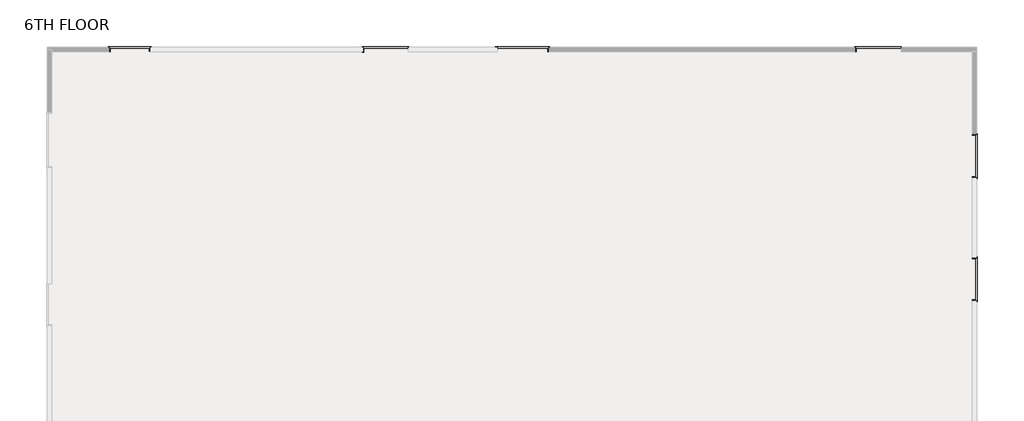
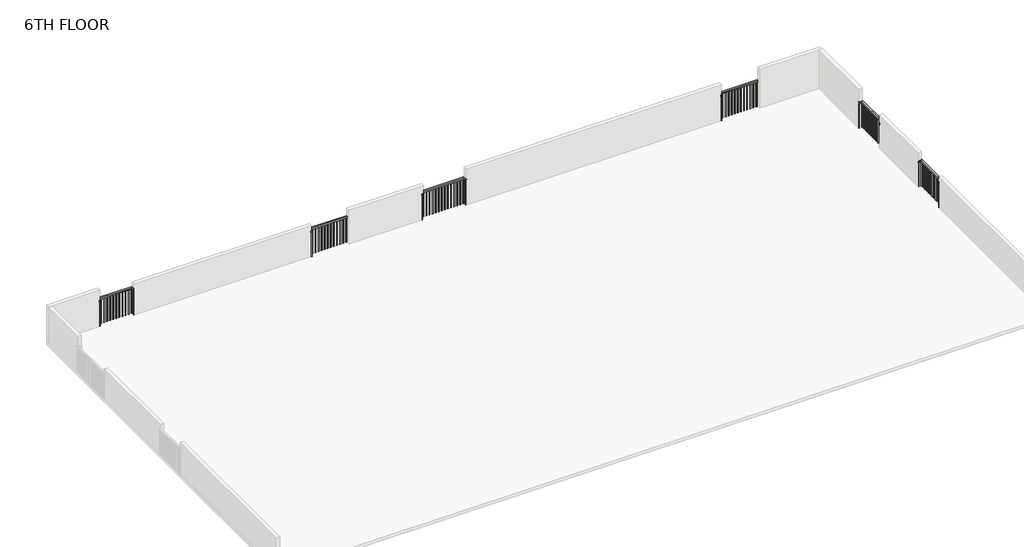
# One storey, part 3 of 3: 6 railings.
"""IFC4 building model written with IfcOpenShell, lengths in millimetres."""

from ifc_helpers import new_model, si_unit, frame, origin, place, context, project, spatial, polyline, outline, extrude, faceted_brep, element, save

model = new_model("IFC4")

# Units and contexts
model_context = context("Model", 3, world=origin())
ifc_project = project(units=[si_unit("LENGTHUNIT", "METRE", prefix="MILLI")], contexts=[model_context])

# Site, building, storey
site = spatial("IfcSite", under=ifc_project)
building = spatial("IfcBuilding", under=site)
storey = spatial("IfcBuildingStorey", under=building, Name="6TH FLOOR", Elevation=19202.4)

# Railings
placement = place(None, origin())
element("IfcRailing", 1, ObjectType="Handrail - Rectangular", at=placement, inside=storey, context=model_context, shape_type="SolidModel", body=[
    faceted_brep([(-11412.4067989, 8355.7067329, 20116.8), (-11412.4067989, 8355.7067329, 20066.0), (-11361.6067989, 8355.7067329, 20066.0), (-11361.6067989, 8355.7067329, 20116.8), (-11412.4067989, 8495.4067329, 20116.8), (-11412.4067989, 8495.4067329, 20066.0), (-11361.6067989, 8444.6067329, 20066.0), (-11361.6067989, 8444.6067329, 20116.8), (-10231.3067989, 8495.4067329, 20116.8), (-10231.3067989, 8495.4067329, 20066.0), (-10282.1067989, 8444.6067329, 20066.0), (-10282.1067989, 8444.6067329, 20116.8), (-10231.3067989, 8368.4067329, 20116.8), (-10282.1067989, 8368.4067329, 20116.8), (-10282.1067989, 8368.4067329, 20066.0), (-10231.3067989, 8368.4067329, 20066.0)], [[[0, 1, 2, 3]], [[1, 0, 4, 5]], [[2, 1, 5, 6]], [[3, 2, 6, 7]], [[0, 3, 7, 4]], [[5, 4, 8, 9]], [[6, 5, 9, 10]], [[7, 6, 10, 11]], [[4, 7, 11, 8]], [[12, 13, 14, 15]], [[9, 8, 12, 15]], [[10, 9, 15, 14]], [[11, 10, 14, 13]], [[8, 11, 13, 12]]]),
    extrude(outline(polyline([(-10278.9317989, 8460.4817329), (-10278.9317989, 8479.5317329), (-10259.8817989, 8479.5317329), (-10259.8817989, 8460.4817329), (-10278.9317989, 8460.4817329)])), frame((0.0, 0.0, 19202.4), z_axis=(0.0, 0.0, 1.0), x_axis=(1.0, 0.0, 0.0)), (0.0, 0.0, 1.0), 863.6),
    extrude(outline(polyline([(-10380.5317989, 8460.4817329), (-10380.5317989, 8479.5317329), (-10361.4817989, 8479.5317329), (-10361.4817989, 8460.4817329), (-10380.5317989, 8460.4817329)])), frame((0.0, 0.0, 19202.4), z_axis=(0.0, 0.0, 1.0), x_axis=(1.0, 0.0, 0.0)), (0.0, 0.0, 1.0), 863.6),
    extrude(outline(polyline([(-10482.1317989, 8460.4817329), (-10482.1317989, 8479.5317329), (-10463.0817989, 8479.5317329), (-10463.0817989, 8460.4817329), (-10482.1317989, 8460.4817329)])), frame((0.0, 0.0, 19202.4), z_axis=(0.0, 0.0, 1.0), x_axis=(1.0, 0.0, 0.0)), (0.0, 0.0, 1.0), 863.6),
    extrude(outline(polyline([(-10583.7317989, 8460.4817329), (-10583.7317989, 8479.5317329), (-10564.6817989, 8479.5317329), (-10564.6817989, 8460.4817329), (-10583.7317989, 8460.4817329)])), frame((0.0, 0.0, 19202.4), z_axis=(0.0, 0.0, 1.0), x_axis=(1.0, 0.0, 0.0)), (0.0, 0.0, 1.0), 863.6),
    extrude(outline(polyline([(-10685.3317989, 8460.4817329), (-10685.3317989, 8479.5317329), (-10666.2817989, 8479.5317329), (-10666.2817989, 8460.4817329), (-10685.3317989, 8460.4817329)])), frame((0.0, 0.0, 19202.4), z_axis=(0.0, 0.0, 1.0), x_axis=(1.0, 0.0, 0.0)), (0.0, 0.0, 1.0), 863.6),
    extrude(outline(polyline([(-10786.9317989, 8460.4817329), (-10786.9317989, 8479.5317329), (-10767.8817989, 8479.5317329), (-10767.8817989, 8460.4817329), (-10786.9317989, 8460.4817329)])), frame((0.0, 0.0, 19202.4), z_axis=(0.0, 0.0, 1.0), x_axis=(1.0, 0.0, 0.0)), (0.0, 0.0, 1.0), 863.6),
    extrude(outline(polyline([(-10888.5317989, 8460.4817329), (-10888.5317989, 8479.5317329), (-10869.4817989, 8479.5317329), (-10869.4817989, 8460.4817329), (-10888.5317989, 8460.4817329)])), frame((0.0, 0.0, 19202.4), z_axis=(0.0, 0.0, 1.0), x_axis=(1.0, 0.0, 0.0)), (0.0, 0.0, 1.0), 863.6),
    extrude(outline(polyline([(-10990.1317989, 8460.4817329), (-10990.1317989, 8479.5317329), (-10971.0817989, 8479.5317329), (-10971.0817989, 8460.4817329), (-10990.1317989, 8460.4817329)])), frame((0.0, 0.0, 19202.4), z_axis=(0.0, 0.0, 1.0), x_axis=(1.0, 0.0, 0.0)), (0.0, 0.0, 1.0), 863.6),
    extrude(outline(polyline([(-11091.7317989, 8460.4817329), (-11091.7317989, 8479.5317329), (-11072.6817989, 8479.5317329), (-11072.6817989, 8460.4817329), (-11091.7317989, 8460.4817329)])), frame((0.0, 0.0, 19202.4), z_axis=(0.0, 0.0, 1.0), x_axis=(1.0, 0.0, 0.0)), (0.0, 0.0, 1.0), 863.6),
    extrude(outline(polyline([(-11193.3317989, 8460.4817329), (-11193.3317989, 8479.5317329), (-11174.2817989, 8479.5317329), (-11174.2817989, 8460.4817329), (-11193.3317989, 8460.4817329)])), frame((0.0, 0.0, 19202.4), z_axis=(0.0, 0.0, 1.0), x_axis=(1.0, 0.0, 0.0)), (0.0, 0.0, 1.0), 863.6),
    extrude(outline(polyline([(-11294.9317989, 8460.4817329), (-11294.9317989, 8479.5317329), (-11275.8817989, 8479.5317329), (-11275.8817989, 8460.4817329), (-11294.9317989, 8460.4817329)])), frame((0.0, 0.0, 19202.4), z_axis=(0.0, 0.0, 1.0), x_axis=(1.0, 0.0, 0.0)), (0.0, 0.0, 1.0), 863.6),
    extrude(outline(polyline([(-11377.4817989, 8447.7817329), (-11396.5317989, 8447.7817329), (-11396.5317989, 8466.8317329), (-11377.4817989, 8466.8317329), (-11377.4817989, 8447.7817329)])), frame((0.0, 0.0, 19202.4), z_axis=(0.0, 0.0, 1.0), x_axis=(1.0, 0.0, 0.0)), (0.0, 0.0, 1.0), 863.6),
    extrude(outline(polyline([(-10266.2317989, 8460.4817329), (-10266.2317989, 8479.5317329), (-10247.1817989, 8479.5317329), (-10247.1817989, 8460.4817329), (-10266.2317989, 8460.4817329)])), frame((0.0, 0.0, 19202.4), z_axis=(0.0, 0.0, 1.0), x_axis=(1.0, 0.0, 0.0)), (0.0, 0.0, 1.0), 863.6),
    extrude(outline(polyline([(-11377.4817989, 8460.4817329), (-11396.5317989, 8460.4817329), (-11396.5317989, 8479.5317329), (-11377.4817989, 8479.5317329), (-11377.4817989, 8460.4817329)])), frame((0.0, 0.0, 19202.4), z_axis=(0.0, 0.0, 1.0), x_axis=(1.0, 0.0, 0.0)), (0.0, 0.0, 1.0), 863.6),
    extrude(outline(polyline([(-10266.2317989, 8387.4567329), (-10247.1817989, 8387.4567329), (-10247.1817989, 8368.4067329), (-10266.2317989, 8368.4067329), (-10266.2317989, 8387.4567329)])), frame((0.0, 0.0, 19202.4), z_axis=(0.0, 0.0, 1.0), x_axis=(1.0, 0.0, 0.0)), (0.0, 0.0, 1.0), 863.6),
    extrude(outline(polyline([(-11377.4817989, 8355.7067329), (-11396.5317989, 8355.7067329), (-11396.5317989, 8374.7567329), (-11377.4817989, 8374.7567329), (-11377.4817989, 8355.7067329)])), frame((0.0, 0.0, 19202.4), z_axis=(0.0, 0.0, 1.0), x_axis=(1.0, 0.0, 0.0)), (0.0, 0.0, 1.0), 863.6),
])
element("IfcRailing", 2, ObjectType="Handrail - Rectangular", at=placement, inside=storey, context=model_context, shape_type="SolidModel", body=[
    faceted_brep([(-4407.8487992, 8336.6567329, 20116.8), (-4407.8487992, 8336.6567329, 20066.0), (-4357.0487992, 8336.6567329, 20066.0), (-4357.0487992, 8336.6567329, 20116.8), (-4407.8487992, 8495.4067329, 20116.8), (-4407.8487992, 8495.4067329, 20066.0), (-4357.0487992, 8444.6067329, 20066.0), (-4357.0487992, 8444.6067329, 20116.8), (-3120.4490672, 8495.4067329, 20116.8), (-3120.4490672, 8444.6067329, 20116.8), (-3120.4490672, 8444.6067329, 20066.0), (-3120.4490672, 8495.4067329, 20066.0)], [[[0, 1, 2, 3]], [[1, 0, 4, 5]], [[2, 1, 5, 6]], [[3, 2, 6, 7]], [[0, 3, 7, 4]], [[8, 9, 10, 11]], [[5, 4, 8, 11]], [[6, 5, 11, 10]], [[7, 6, 10, 9]], [[4, 7, 9, 8]]]),
    extrude(outline(polyline([(-3172.7737992, 8460.4817329), (-3172.7737992, 8479.5317329), (-3153.7237992, 8479.5317329), (-3153.7237992, 8460.4817329), (-3172.7737992, 8460.4817329)])), frame((0.0, 0.0, 19202.4), z_axis=(0.0, 0.0, 1.0), x_axis=(1.0, 0.0, 0.0)), (0.0, 0.0, 1.0), 863.6),
    extrude(outline(polyline([(-3274.3737992, 8460.4817329), (-3274.3737992, 8479.5317329), (-3255.3237992, 8479.5317329), (-3255.3237992, 8460.4817329), (-3274.3737992, 8460.4817329)])), frame((0.0, 0.0, 19202.4), z_axis=(0.0, 0.0, 1.0), x_axis=(1.0, 0.0, 0.0)), (0.0, 0.0, 1.0), 863.6),
    extrude(outline(polyline([(-3375.9737992, 8460.4817329), (-3375.9737992, 8479.5317329), (-3356.9237992, 8479.5317329), (-3356.9237992, 8460.4817329), (-3375.9737992, 8460.4817329)])), frame((0.0, 0.0, 19202.4), z_axis=(0.0, 0.0, 1.0), x_axis=(1.0, 0.0, 0.0)), (0.0, 0.0, 1.0), 863.6),
    extrude(outline(polyline([(-3477.5737992, 8460.4817329), (-3477.5737992, 8479.5317329), (-3458.5237992, 8479.5317329), (-3458.5237992, 8460.4817329), (-3477.5737992, 8460.4817329)])), frame((0.0, 0.0, 19202.4), z_axis=(0.0, 0.0, 1.0), x_axis=(1.0, 0.0, 0.0)), (0.0, 0.0, 1.0), 863.6),
    extrude(outline(polyline([(-3579.1737992, 8460.4817329), (-3579.1737992, 8479.5317329), (-3560.1237992, 8479.5317329), (-3560.1237992, 8460.4817329), (-3579.1737992, 8460.4817329)])), frame((0.0, 0.0, 19202.4), z_axis=(0.0, 0.0, 1.0), x_axis=(1.0, 0.0, 0.0)), (0.0, 0.0, 1.0), 863.6),
    extrude(outline(polyline([(-3680.7737992, 8460.4817329), (-3680.7737992, 8479.5317329), (-3661.7237992, 8479.5317329), (-3661.7237992, 8460.4817329), (-3680.7737992, 8460.4817329)])), frame((0.0, 0.0, 19202.4), z_axis=(0.0, 0.0, 1.0), x_axis=(1.0, 0.0, 0.0)), (0.0, 0.0, 1.0), 863.6),
    extrude(outline(polyline([(-3782.3737992, 8460.4817329), (-3782.3737992, 8479.5317329), (-3763.3237992, 8479.5317329), (-3763.3237992, 8460.4817329), (-3782.3737992, 8460.4817329)])), frame((0.0, 0.0, 19202.4), z_axis=(0.0, 0.0, 1.0), x_axis=(1.0, 0.0, 0.0)), (0.0, 0.0, 1.0), 863.6),
    extrude(outline(polyline([(-3883.9737992, 8460.4817329), (-3883.9737992, 8479.5317329), (-3864.9237992, 8479.5317329), (-3864.9237992, 8460.4817329), (-3883.9737992, 8460.4817329)])), frame((0.0, 0.0, 19202.4), z_axis=(0.0, 0.0, 1.0), x_axis=(1.0, 0.0, 0.0)), (0.0, 0.0, 1.0), 863.6),
    extrude(outline(polyline([(-3985.5737992, 8460.4817329), (-3985.5737992, 8479.5317329), (-3966.5237992, 8479.5317329), (-3966.5237992, 8460.4817329), (-3985.5737992, 8460.4817329)])), frame((0.0, 0.0, 19202.4), z_axis=(0.0, 0.0, 1.0), x_axis=(1.0, 0.0, 0.0)), (0.0, 0.0, 1.0), 863.6),
    extrude(outline(polyline([(-4087.1737992, 8460.4817329), (-4087.1737992, 8479.5317329), (-4068.1237992, 8479.5317329), (-4068.1237992, 8460.4817329), (-4087.1737992, 8460.4817329)])), frame((0.0, 0.0, 19202.4), z_axis=(0.0, 0.0, 1.0), x_axis=(1.0, 0.0, 0.0)), (0.0, 0.0, 1.0), 863.6),
    extrude(outline(polyline([(-4188.7737992, 8460.4817329), (-4188.7737992, 8479.5317329), (-4169.7237992, 8479.5317329), (-4169.7237992, 8460.4817329), (-4188.7737992, 8460.4817329)])), frame((0.0, 0.0, 19202.4), z_axis=(0.0, 0.0, 1.0), x_axis=(1.0, 0.0, 0.0)), (0.0, 0.0, 1.0), 863.6),
    extrude(outline(polyline([(-4290.3737992, 8460.4817329), (-4290.3737992, 8479.5317329), (-4271.3237992, 8479.5317329), (-4271.3237992, 8460.4817329), (-4290.3737992, 8460.4817329)])), frame((0.0, 0.0, 19202.4), z_axis=(0.0, 0.0, 1.0), x_axis=(1.0, 0.0, 0.0)), (0.0, 0.0, 1.0), 863.6),
    extrude(outline(polyline([(-4372.9237992, 8428.7317329), (-4391.9737992, 8428.7317329), (-4391.9737992, 8447.7817329), (-4372.9237992, 8447.7817329), (-4372.9237992, 8428.7317329)])), frame((0.0, 0.0, 19202.4), z_axis=(0.0, 0.0, 1.0), x_axis=(1.0, 0.0, 0.0)), (0.0, 0.0, 1.0), 863.6),
    extrude(outline(polyline([(-4372.9237992, 8460.4817329), (-4391.9737992, 8460.4817329), (-4391.9737992, 8479.5317329), (-4372.9237992, 8479.5317329), (-4372.9237992, 8460.4817329)])), frame((0.0, 0.0, 19202.4), z_axis=(0.0, 0.0, 1.0), x_axis=(1.0, 0.0, 0.0)), (0.0, 0.0, 1.0), 863.6),
    extrude(outline(polyline([(-3139.4990672, 8460.4817329), (-3139.4990672, 8479.5317329), (-3120.4490672, 8479.5317329), (-3120.4490672, 8460.4817329), (-3139.4990672, 8460.4817329)])), frame((0.0, 0.0, 19202.4), z_axis=(0.0, 0.0, 1.0), x_axis=(1.0, 0.0, 0.0)), (0.0, 0.0, 1.0), 863.6),
    extrude(outline(polyline([(-4372.9237992, 8336.6567329), (-4391.9737992, 8336.6567329), (-4391.9737992, 8355.7067329), (-4372.9237992, 8355.7067329), (-4372.9237992, 8336.6567329)])), frame((0.0, 0.0, 19202.4), z_axis=(0.0, 0.0, 1.0), x_axis=(1.0, 0.0, 0.0)), (0.0, 0.0, 1.0), 863.6),
])
element("IfcRailing", 3, ObjectType="Handrail - Rectangular", at=placement, inside=storey, context=model_context, shape_type="SolidModel", body=[
    faceted_brep([(-732.8490672, 8355.7067329, 20116.8), (-732.8490672, 8355.7067329, 20066.0), (-682.0490672, 8355.7067329, 20066.0), (-682.0490672, 8355.7067329, 20116.8), (-732.8490672, 8495.4067329, 20116.8), (-732.8490672, 8495.4067329, 20066.0), (-682.0490672, 8444.6067329, 20066.0), (-682.0490672, 8444.6067329, 20116.8), (766.8932011, 8495.4067329, 20116.8), (766.8932011, 8495.4067329, 20066.0), (716.0932011, 8444.6067329, 20066.0), (716.0932011, 8444.6067329, 20116.8), (766.8932011, 8355.7067329, 20116.8), (716.0932011, 8355.7067329, 20116.8), (716.0932011, 8355.7067329, 20066.0), (766.8932011, 8355.7067329, 20066.0)], [[[0, 1, 2, 3]], [[1, 0, 4, 5]], [[2, 1, 5, 6]], [[3, 2, 6, 7]], [[0, 3, 7, 4]], [[5, 4, 8, 9]], [[6, 5, 9, 10]], [[7, 6, 10, 11]], [[4, 7, 11, 8]], [[12, 13, 14, 15]], [[9, 8, 12, 15]], [[10, 9, 15, 14]], [[11, 10, 14, 13]], [[8, 11, 13, 12]]]),
    extrude(outline(polyline([(731.9682011, 8377.9317329), (751.0182011, 8377.9317329), (751.0182011, 8358.8817329), (731.9682011, 8358.8817329), (731.9682011, 8377.9317329)])), frame((0.0, 0.0, 19202.4), z_axis=(0.0, 0.0, 1.0), x_axis=(1.0, 0.0, 0.0)), (0.0, 0.0, 1.0), 863.6),
    extrude(outline(polyline([(705.4259328, 8460.4817329), (705.4259328, 8479.5317329), (724.4759328, 8479.5317329), (724.4759328, 8460.4817329), (705.4259328, 8460.4817329)])), frame((0.0, 0.0, 19202.4), z_axis=(0.0, 0.0, 1.0), x_axis=(1.0, 0.0, 0.0)), (0.0, 0.0, 1.0), 863.6),
    extrude(outline(polyline([(603.8259328, 8460.4817329), (603.8259328, 8479.5317329), (622.8759328, 8479.5317329), (622.8759328, 8460.4817329), (603.8259328, 8460.4817329)])), frame((0.0, 0.0, 19202.4), z_axis=(0.0, 0.0, 1.0), x_axis=(1.0, 0.0, 0.0)), (0.0, 0.0, 1.0), 863.6),
    extrude(outline(polyline([(502.2259328, 8460.4817329), (502.2259328, 8479.5317329), (521.2759328, 8479.5317329), (521.2759328, 8460.4817329), (502.2259328, 8460.4817329)])), frame((0.0, 0.0, 19202.4), z_axis=(0.0, 0.0, 1.0), x_axis=(1.0, 0.0, 0.0)), (0.0, 0.0, 1.0), 863.6),
    extrude(outline(polyline([(400.6259328, 8460.4817329), (400.6259328, 8479.5317329), (419.6759328, 8479.5317329), (419.6759328, 8460.4817329), (400.6259328, 8460.4817329)])), frame((0.0, 0.0, 19202.4), z_axis=(0.0, 0.0, 1.0), x_axis=(1.0, 0.0, 0.0)), (0.0, 0.0, 1.0), 863.6),
    extrude(outline(polyline([(299.0259328, 8460.4817329), (299.0259328, 8479.5317329), (318.0759328, 8479.5317329), (318.0759328, 8460.4817329), (299.0259328, 8460.4817329)])), frame((0.0, 0.0, 19202.4), z_axis=(0.0, 0.0, 1.0), x_axis=(1.0, 0.0, 0.0)), (0.0, 0.0, 1.0), 863.6),
    extrude(outline(polyline([(197.4259328, 8460.4817329), (197.4259328, 8479.5317329), (216.4759328, 8479.5317329), (216.4759328, 8460.4817329), (197.4259328, 8460.4817329)])), frame((0.0, 0.0, 19202.4), z_axis=(0.0, 0.0, 1.0), x_axis=(1.0, 0.0, 0.0)), (0.0, 0.0, 1.0), 863.6),
    extrude(outline(polyline([(95.8259328, 8460.4817329), (95.8259328, 8479.5317329), (114.8759328, 8479.5317329), (114.8759328, 8460.4817329), (95.8259328, 8460.4817329)])), frame((0.0, 0.0, 19202.4), z_axis=(0.0, 0.0, 1.0), x_axis=(1.0, 0.0, 0.0)), (0.0, 0.0, 1.0), 863.6),
    extrude(outline(polyline([(-5.7740672, 8460.4817329), (-5.7740672, 8479.5317329), (13.2759328, 8479.5317329), (13.2759328, 8460.4817329), (-5.7740672, 8460.4817329)])), frame((0.0, 0.0, 19202.4), z_axis=(0.0, 0.0, 1.0), x_axis=(1.0, 0.0, 0.0)), (0.0, 0.0, 1.0), 863.6),
    extrude(outline(polyline([(-107.3740672, 8460.4817329), (-107.3740672, 8479.5317329), (-88.3240672, 8479.5317329), (-88.3240672, 8460.4817329), (-107.3740672, 8460.4817329)])), frame((0.0, 0.0, 19202.4), z_axis=(0.0, 0.0, 1.0), x_axis=(1.0, 0.0, 0.0)), (0.0, 0.0, 1.0), 863.6),
    extrude(outline(polyline([(-208.9740672, 8460.4817329), (-208.9740672, 8479.5317329), (-189.9240672, 8479.5317329), (-189.9240672, 8460.4817329), (-208.9740672, 8460.4817329)])), frame((0.0, 0.0, 19202.4), z_axis=(0.0, 0.0, 1.0), x_axis=(1.0, 0.0, 0.0)), (0.0, 0.0, 1.0), 863.6),
    extrude(outline(polyline([(-310.5740672, 8460.4817329), (-310.5740672, 8479.5317329), (-291.5240672, 8479.5317329), (-291.5240672, 8460.4817329), (-310.5740672, 8460.4817329)])), frame((0.0, 0.0, 19202.4), z_axis=(0.0, 0.0, 1.0), x_axis=(1.0, 0.0, 0.0)), (0.0, 0.0, 1.0), 863.6),
    extrude(outline(polyline([(-412.1740672, 8460.4817329), (-412.1740672, 8479.5317329), (-393.1240672, 8479.5317329), (-393.1240672, 8460.4817329), (-412.1740672, 8460.4817329)])), frame((0.0, 0.0, 19202.4), z_axis=(0.0, 0.0, 1.0), x_axis=(1.0, 0.0, 0.0)), (0.0, 0.0, 1.0), 863.6),
    extrude(outline(polyline([(-513.7740672, 8460.4817329), (-513.7740672, 8479.5317329), (-494.7240672, 8479.5317329), (-494.7240672, 8460.4817329), (-513.7740672, 8460.4817329)])), frame((0.0, 0.0, 19202.4), z_axis=(0.0, 0.0, 1.0), x_axis=(1.0, 0.0, 0.0)), (0.0, 0.0, 1.0), 863.6),
    extrude(outline(polyline([(-615.3740672, 8460.4817329), (-615.3740672, 8479.5317329), (-596.3240672, 8479.5317329), (-596.3240672, 8460.4817329), (-615.3740672, 8460.4817329)])), frame((0.0, 0.0, 19202.4), z_axis=(0.0, 0.0, 1.0), x_axis=(1.0, 0.0, 0.0)), (0.0, 0.0, 1.0), 863.6),
    extrude(outline(polyline([(-697.9240672, 8447.7817329), (-716.9740672, 8447.7817329), (-716.9740672, 8466.8317329), (-697.9240672, 8466.8317329), (-697.9240672, 8447.7817329)])), frame((0.0, 0.0, 19202.4), z_axis=(0.0, 0.0, 1.0), x_axis=(1.0, 0.0, 0.0)), (0.0, 0.0, 1.0), 863.6),
    extrude(outline(polyline([(731.9682011, 8460.4817329), (731.9682011, 8479.5317329), (751.0182011, 8479.5317329), (751.0182011, 8460.4817329), (731.9682011, 8460.4817329)])), frame((0.0, 0.0, 19202.4), z_axis=(0.0, 0.0, 1.0), x_axis=(1.0, 0.0, 0.0)), (0.0, 0.0, 1.0), 863.6),
    extrude(outline(polyline([(-697.9240672, 8460.4817329), (-716.9740672, 8460.4817329), (-716.9740672, 8479.5317329), (-697.9240672, 8479.5317329), (-697.9240672, 8460.4817329)])), frame((0.0, 0.0, 19202.4), z_axis=(0.0, 0.0, 1.0), x_axis=(1.0, 0.0, 0.0)), (0.0, 0.0, 1.0), 863.6),
    extrude(outline(polyline([(731.9682011, 8374.7567329), (751.0182011, 8374.7567329), (751.0182011, 8355.7067329), (731.9682011, 8355.7067329), (731.9682011, 8374.7567329)])), frame((0.0, 0.0, 19202.4), z_axis=(0.0, 0.0, 1.0), x_axis=(1.0, 0.0, 0.0)), (0.0, 0.0, 1.0), 863.6),
    extrude(outline(polyline([(-697.9240672, 8355.7067329), (-716.9740672, 8355.7067329), (-716.9740672, 8374.7567329), (-697.9240672, 8374.7567329), (-697.9240672, 8355.7067329)])), frame((0.0, 0.0, 19202.4), z_axis=(0.0, 0.0, 1.0), x_axis=(1.0, 0.0, 0.0)), (0.0, 0.0, 1.0), 863.6),
])
element("IfcRailing", 4, ObjectType="Handrail - Rectangular", at=placement, inside=storey, context=model_context, shape_type="SolidModel", body=[
    faceted_brep([(9174.2932011, 8355.7067329, 20116.8), (9174.2932011, 8355.7067329, 20066.0), (9225.0932011, 8355.7067329, 20066.0), (9225.0932011, 8355.7067329, 20116.8), (9174.2932011, 8495.4067329, 20116.8), (9174.2932011, 8495.4067329, 20066.0), (9225.0932011, 8444.6067329, 20066.0), (9225.0932011, 8444.6067329, 20116.8), (10462.2009401, 8495.4067329, 20116.8), (10462.2009401, 8444.6067329, 20116.8), (10462.2009401, 8444.6067329, 20066.0), (10462.2009401, 8495.4067329, 20066.0)], [[[0, 1, 2, 3]], [[1, 0, 4, 5]], [[2, 1, 5, 6]], [[3, 2, 6, 7]], [[0, 3, 7, 4]], [[8, 9, 10, 11]], [[5, 4, 8, 11]], [[6, 5, 11, 10]], [[7, 6, 10, 9]], [[4, 7, 9, 8]]]),
    extrude(outline(polyline([(10409.3682011, 8460.4817329), (10409.3682011, 8479.5317329), (10428.4182011, 8479.5317329), (10428.4182011, 8460.4817329), (10409.3682011, 8460.4817329)])), frame((0.0, 0.0, 19202.4), z_axis=(0.0, 0.0, 1.0), x_axis=(1.0, 0.0, 0.0)), (0.0, 0.0, 1.0), 863.6),
    extrude(outline(polyline([(10307.7682011, 8460.4817329), (10307.7682011, 8479.5317329), (10326.8182011, 8479.5317329), (10326.8182011, 8460.4817329), (10307.7682011, 8460.4817329)])), frame((0.0, 0.0, 19202.4), z_axis=(0.0, 0.0, 1.0), x_axis=(1.0, 0.0, 0.0)), (0.0, 0.0, 1.0), 863.6),
    extrude(outline(polyline([(10206.1682011, 8460.4817329), (10206.1682011, 8479.5317329), (10225.2182011, 8479.5317329), (10225.2182011, 8460.4817329), (10206.1682011, 8460.4817329)])), frame((0.0, 0.0, 19202.4), z_axis=(0.0, 0.0, 1.0), x_axis=(1.0, 0.0, 0.0)), (0.0, 0.0, 1.0), 863.6),
    extrude(outline(polyline([(10104.5682011, 8460.4817329), (10104.5682011, 8479.5317329), (10123.6182011, 8479.5317329), (10123.6182011, 8460.4817329), (10104.5682011, 8460.4817329)])), frame((0.0, 0.0, 19202.4), z_axis=(0.0, 0.0, 1.0), x_axis=(1.0, 0.0, 0.0)), (0.0, 0.0, 1.0), 863.6),
    extrude(outline(polyline([(10002.9682011, 8460.4817329), (10002.9682011, 8479.5317329), (10022.0182011, 8479.5317329), (10022.0182011, 8460.4817329), (10002.9682011, 8460.4817329)])), frame((0.0, 0.0, 19202.4), z_axis=(0.0, 0.0, 1.0), x_axis=(1.0, 0.0, 0.0)), (0.0, 0.0, 1.0), 863.6),
    extrude(outline(polyline([(9901.3682011, 8460.4817329), (9901.3682011, 8479.5317329), (9920.4182011, 8479.5317329), (9920.4182011, 8460.4817329), (9901.3682011, 8460.4817329)])), frame((0.0, 0.0, 19202.4), z_axis=(0.0, 0.0, 1.0), x_axis=(1.0, 0.0, 0.0)), (0.0, 0.0, 1.0), 863.6),
    extrude(outline(polyline([(9799.7682011, 8460.4817329), (9799.7682011, 8479.5317329), (9818.8182011, 8479.5317329), (9818.8182011, 8460.4817329), (9799.7682011, 8460.4817329)])), frame((0.0, 0.0, 19202.4), z_axis=(0.0, 0.0, 1.0), x_axis=(1.0, 0.0, 0.0)), (0.0, 0.0, 1.0), 863.6),
    extrude(outline(polyline([(9698.1682011, 8460.4817329), (9698.1682011, 8479.5317329), (9717.2182011, 8479.5317329), (9717.2182011, 8460.4817329), (9698.1682011, 8460.4817329)])), frame((0.0, 0.0, 19202.4), z_axis=(0.0, 0.0, 1.0), x_axis=(1.0, 0.0, 0.0)), (0.0, 0.0, 1.0), 863.6),
    extrude(outline(polyline([(9596.5682011, 8460.4817329), (9596.5682011, 8479.5317329), (9615.6182011, 8479.5317329), (9615.6182011, 8460.4817329), (9596.5682011, 8460.4817329)])), frame((0.0, 0.0, 19202.4), z_axis=(0.0, 0.0, 1.0), x_axis=(1.0, 0.0, 0.0)), (0.0, 0.0, 1.0), 863.6),
    extrude(outline(polyline([(9494.9682011, 8460.4817329), (9494.9682011, 8479.5317329), (9514.0182011, 8479.5317329), (9514.0182011, 8460.4817329), (9494.9682011, 8460.4817329)])), frame((0.0, 0.0, 19202.4), z_axis=(0.0, 0.0, 1.0), x_axis=(1.0, 0.0, 0.0)), (0.0, 0.0, 1.0), 863.6),
    extrude(outline(polyline([(9393.3682011, 8460.4817329), (9393.3682011, 8479.5317329), (9412.4182011, 8479.5317329), (9412.4182011, 8460.4817329), (9393.3682011, 8460.4817329)])), frame((0.0, 0.0, 19202.4), z_axis=(0.0, 0.0, 1.0), x_axis=(1.0, 0.0, 0.0)), (0.0, 0.0, 1.0), 863.6),
    extrude(outline(polyline([(9291.7682011, 8460.4817329), (9291.7682011, 8479.5317329), (9310.8182011, 8479.5317329), (9310.8182011, 8460.4817329), (9291.7682011, 8460.4817329)])), frame((0.0, 0.0, 19202.4), z_axis=(0.0, 0.0, 1.0), x_axis=(1.0, 0.0, 0.0)), (0.0, 0.0, 1.0), 863.6),
    extrude(outline(polyline([(9209.2182011, 8447.7817329), (9190.1682011, 8447.7817329), (9190.1682011, 8466.8317329), (9209.2182011, 8466.8317329), (9209.2182011, 8447.7817329)])), frame((0.0, 0.0, 19202.4), z_axis=(0.0, 0.0, 1.0), x_axis=(1.0, 0.0, 0.0)), (0.0, 0.0, 1.0), 863.6),
    extrude(outline(polyline([(9209.2182011, 8460.4817329), (9190.1682011, 8460.4817329), (9190.1682011, 8479.5317329), (9209.2182011, 8479.5317329), (9209.2182011, 8460.4817329)])), frame((0.0, 0.0, 19202.4), z_axis=(0.0, 0.0, 1.0), x_axis=(1.0, 0.0, 0.0)), (0.0, 0.0, 1.0), 863.6),
    extrude(outline(polyline([(10443.1509401, 8460.4817329), (10443.1509401, 8479.5317329), (10462.2009401, 8479.5317329), (10462.2009401, 8460.4817329), (10443.1509401, 8460.4817329)])), frame((0.0, 0.0, 19202.4), z_axis=(0.0, 0.0, 1.0), x_axis=(1.0, 0.0, 0.0)), (0.0, 0.0, 1.0), 863.6),
    extrude(outline(polyline([(9209.2182011, 8355.7067329), (9190.1682011, 8355.7067329), (9190.1682011, 8374.7567329), (9209.2182011, 8374.7567329), (9209.2182011, 8355.7067329)])), frame((0.0, 0.0, 19202.4), z_axis=(0.0, 0.0, 1.0), x_axis=(1.0, 0.0, 0.0)), (0.0, 0.0, 1.0), 863.6),
])
element("IfcRailing", 5, ObjectType="Handrail - Rectangular", at=placement, inside=storey, context=model_context, shape_type="SolidModel", body=[
    faceted_brep([(12426.0012043, 2691.5067329, 20116.8), (12426.0012043, 2691.5067329, 20066.0), (12426.0012043, 2640.7067329, 20066.0), (12426.0012043, 2640.7067329, 20116.8), (12565.7012043, 2691.5067329, 20116.8), (12565.7012043, 2691.5067329, 20066.0), (12514.9012043, 2640.7067329, 20066.0), (12514.9012043, 2640.7067329, 20116.8), (12565.7012043, 1453.2567334, 20116.8), (12565.7012043, 1453.2567334, 20066.0), (12514.9012043, 1504.0567334, 20066.0), (12514.9012043, 1504.0567334, 20116.8), (12426.0012043, 1453.2567334, 20116.8), (12426.0012043, 1504.0567334, 20116.8), (12426.0012043, 1504.0567334, 20066.0), (12426.0012043, 1453.2567334, 20066.0)], [[[0, 1, 2, 3]], [[1, 0, 4, 5]], [[2, 1, 5, 6]], [[3, 2, 6, 7]], [[0, 3, 7, 4]], [[5, 4, 8, 9]], [[6, 5, 9, 10]], [[7, 6, 10, 11]], [[4, 7, 11, 8]], [[12, 13, 14, 15]], [[9, 8, 12, 15]], [[10, 9, 15, 14]], [[11, 10, 14, 13]], [[8, 11, 13, 12]]]),
    extrude(outline(polyline([(12448.2262043, 1488.1817334), (12448.2262043, 1469.1317334), (12429.1762043, 1469.1317334), (12429.1762043, 1488.1817334), (12448.2262043, 1488.1817334)])), frame((0.0, 0.0, 19202.4), z_axis=(0.0, 0.0, 1.0), x_axis=(1.0, 0.0, 0.0)), (0.0, 0.0, 1.0), 863.6),
    extrude(outline(polyline([(12530.7762043, 1558.0317329), (12549.8262043, 1558.0317329), (12549.8262043, 1538.9817329), (12530.7762043, 1538.9817329), (12530.7762043, 1558.0317329)])), frame((0.0, 0.0, 19202.4), z_axis=(0.0, 0.0, 1.0), x_axis=(1.0, 0.0, 0.0)), (0.0, 0.0, 1.0), 863.6),
    extrude(outline(polyline([(12530.7762043, 1659.6317329), (12549.8262043, 1659.6317329), (12549.8262043, 1640.5817329), (12530.7762043, 1640.5817329), (12530.7762043, 1659.6317329)])), frame((0.0, 0.0, 19202.4), z_axis=(0.0, 0.0, 1.0), x_axis=(1.0, 0.0, 0.0)), (0.0, 0.0, 1.0), 863.6),
    extrude(outline(polyline([(12530.7762043, 1761.2317329), (12549.8262043, 1761.2317329), (12549.8262043, 1742.1817329), (12530.7762043, 1742.1817329), (12530.7762043, 1761.2317329)])), frame((0.0, 0.0, 19202.4), z_axis=(0.0, 0.0, 1.0), x_axis=(1.0, 0.0, 0.0)), (0.0, 0.0, 1.0), 863.6),
    extrude(outline(polyline([(12530.7762043, 1862.8317329), (12549.8262043, 1862.8317329), (12549.8262043, 1843.7817329), (12530.7762043, 1843.7817329), (12530.7762043, 1862.8317329)])), frame((0.0, 0.0, 19202.4), z_axis=(0.0, 0.0, 1.0), x_axis=(1.0, 0.0, 0.0)), (0.0, 0.0, 1.0), 863.6),
    extrude(outline(polyline([(12530.7762043, 1964.4317329), (12549.8262043, 1964.4317329), (12549.8262043, 1945.3817329), (12530.7762043, 1945.3817329), (12530.7762043, 1964.4317329)])), frame((0.0, 0.0, 19202.4), z_axis=(0.0, 0.0, 1.0), x_axis=(1.0, 0.0, 0.0)), (0.0, 0.0, 1.0), 863.6),
    extrude(outline(polyline([(12530.7762043, 2066.0317329), (12549.8262043, 2066.0317329), (12549.8262043, 2046.9817329), (12530.7762043, 2046.9817329), (12530.7762043, 2066.0317329)])), frame((0.0, 0.0, 19202.4), z_axis=(0.0, 0.0, 1.0), x_axis=(1.0, 0.0, 0.0)), (0.0, 0.0, 1.0), 863.6),
    extrude(outline(polyline([(12530.7762043, 2167.6317329), (12549.8262043, 2167.6317329), (12549.8262043, 2148.5817329), (12530.7762043, 2148.5817329), (12530.7762043, 2167.6317329)])), frame((0.0, 0.0, 19202.4), z_axis=(0.0, 0.0, 1.0), x_axis=(1.0, 0.0, 0.0)), (0.0, 0.0, 1.0), 863.6),
    extrude(outline(polyline([(12530.7762043, 2269.2317329), (12549.8262043, 2269.2317329), (12549.8262043, 2250.1817329), (12530.7762043, 2250.1817329), (12530.7762043, 2269.2317329)])), frame((0.0, 0.0, 19202.4), z_axis=(0.0, 0.0, 1.0), x_axis=(1.0, 0.0, 0.0)), (0.0, 0.0, 1.0), 863.6),
    extrude(outline(polyline([(12530.7762043, 2370.8317329), (12549.8262043, 2370.8317329), (12549.8262043, 2351.7817329), (12530.7762043, 2351.7817329), (12530.7762043, 2370.8317329)])), frame((0.0, 0.0, 19202.4), z_axis=(0.0, 0.0, 1.0), x_axis=(1.0, 0.0, 0.0)), (0.0, 0.0, 1.0), 863.6),
    extrude(outline(polyline([(12530.7762043, 2472.4317329), (12549.8262043, 2472.4317329), (12549.8262043, 2453.3817329), (12530.7762043, 2453.3817329), (12530.7762043, 2472.4317329)])), frame((0.0, 0.0, 19202.4), z_axis=(0.0, 0.0, 1.0), x_axis=(1.0, 0.0, 0.0)), (0.0, 0.0, 1.0), 863.6),
    extrude(outline(polyline([(12530.7762043, 2574.0317329), (12549.8262043, 2574.0317329), (12549.8262043, 2554.9817329), (12530.7762043, 2554.9817329), (12530.7762043, 2574.0317329)])), frame((0.0, 0.0, 19202.4), z_axis=(0.0, 0.0, 1.0), x_axis=(1.0, 0.0, 0.0)), (0.0, 0.0, 1.0), 863.6),
    extrude(outline(polyline([(12518.0762043, 2656.5817329), (12518.0762043, 2675.6317329), (12537.1262043, 2675.6317329), (12537.1262043, 2656.5817329), (12518.0762043, 2656.5817329)])), frame((0.0, 0.0, 19202.4), z_axis=(0.0, 0.0, 1.0), x_axis=(1.0, 0.0, 0.0)), (0.0, 0.0, 1.0), 863.6),
    extrude(outline(polyline([(12530.7762043, 1488.1817334), (12549.8262043, 1488.1817334), (12549.8262043, 1469.1317334), (12530.7762043, 1469.1317334), (12530.7762043, 1488.1817334)])), frame((0.0, 0.0, 19202.4), z_axis=(0.0, 0.0, 1.0), x_axis=(1.0, 0.0, 0.0)), (0.0, 0.0, 1.0), 863.6),
    extrude(outline(polyline([(12530.7762043, 2656.5817329), (12530.7762043, 2675.6317329), (12549.8262043, 2675.6317329), (12549.8262043, 2656.5817329), (12530.7762043, 2656.5817329)])), frame((0.0, 0.0, 19202.4), z_axis=(0.0, 0.0, 1.0), x_axis=(1.0, 0.0, 0.0)), (0.0, 0.0, 1.0), 863.6),
    extrude(outline(polyline([(12445.0512043, 1488.1817334), (12445.0512043, 1469.1317334), (12426.0012043, 1469.1317334), (12426.0012043, 1488.1817334), (12445.0512043, 1488.1817334)])), frame((0.0, 0.0, 19202.4), z_axis=(0.0, 0.0, 1.0), x_axis=(1.0, 0.0, 0.0)), (0.0, 0.0, 1.0), 863.6),
    extrude(outline(polyline([(12426.0012043, 2656.5817329), (12426.0012043, 2675.6317329), (12445.0512043, 2675.6317329), (12445.0512043, 2656.5817329), (12426.0012043, 2656.5817329)])), frame((0.0, 0.0, 19202.4), z_axis=(0.0, 0.0, 1.0), x_axis=(1.0, 0.0, 0.0)), (0.0, 0.0, 1.0), 863.6),
])
element("IfcRailing", 6, ObjectType="Handrail - Rectangular", at=placement, inside=storey, context=model_context, shape_type="SolidModel", body=[
    faceted_brep([(12426.0012043, 6095.1067329, 20116.8), (12426.0012043, 6095.1067329, 20066.0), (12426.0012043, 6044.3067329, 20066.0), (12426.0012043, 6044.3067329, 20116.8), (12565.7012043, 6095.1067329, 20116.8), (12565.7012043, 6095.1067329, 20066.0), (12514.9012043, 6044.3067329, 20066.0), (12514.9012043, 6044.3067329, 20116.8), (12565.7012043, 4850.5067329, 20116.8), (12565.7012043, 4850.5067329, 20066.0), (12514.9012043, 4901.3067329, 20066.0), (12514.9012043, 4901.3067329, 20116.8), (12426.0012043, 4850.5067329, 20116.8), (12426.0012043, 4901.3067329, 20116.8), (12426.0012043, 4901.3067329, 20066.0), (12426.0012043, 4850.5067329, 20066.0)], [[[0, 1, 2, 3]], [[1, 0, 4, 5]], [[2, 1, 5, 6]], [[3, 2, 6, 7]], [[0, 3, 7, 4]], [[5, 4, 8, 9]], [[6, 5, 9, 10]], [[7, 6, 10, 11]], [[4, 7, 11, 8]], [[12, 13, 14, 15]], [[9, 8, 12, 15]], [[10, 9, 15, 14]], [[11, 10, 14, 13]], [[8, 11, 13, 12]]]),
    extrude(outline(polyline([(12448.2262043, 4885.4317329), (12448.2262043, 4866.3817329), (12429.1762043, 4866.3817329), (12429.1762043, 4885.4317329), (12448.2262043, 4885.4317329)])), frame((0.0, 0.0, 19202.4), z_axis=(0.0, 0.0, 1.0), x_axis=(1.0, 0.0, 0.0)), (0.0, 0.0, 1.0), 863.6),
    extrude(outline(polyline([(12530.7762043, 4961.6317329), (12549.8262043, 4961.6317329), (12549.8262043, 4942.5817329), (12530.7762043, 4942.5817329), (12530.7762043, 4961.6317329)])), frame((0.0, 0.0, 19202.4), z_axis=(0.0, 0.0, 1.0), x_axis=(1.0, 0.0, 0.0)), (0.0, 0.0, 1.0), 863.6),
    extrude(outline(polyline([(12530.7762043, 5063.2317329), (12549.8262043, 5063.2317329), (12549.8262043, 5044.1817329), (12530.7762043, 5044.1817329), (12530.7762043, 5063.2317329)])), frame((0.0, 0.0, 19202.4), z_axis=(0.0, 0.0, 1.0), x_axis=(1.0, 0.0, 0.0)), (0.0, 0.0, 1.0), 863.6),
    extrude(outline(polyline([(12530.7762043, 5164.8317329), (12549.8262043, 5164.8317329), (12549.8262043, 5145.7817329), (12530.7762043, 5145.7817329), (12530.7762043, 5164.8317329)])), frame((0.0, 0.0, 19202.4), z_axis=(0.0, 0.0, 1.0), x_axis=(1.0, 0.0, 0.0)), (0.0, 0.0, 1.0), 863.6),
    extrude(outline(polyline([(12530.7762043, 5266.4317329), (12549.8262043, 5266.4317329), (12549.8262043, 5247.3817329), (12530.7762043, 5247.3817329), (12530.7762043, 5266.4317329)])), frame((0.0, 0.0, 19202.4), z_axis=(0.0, 0.0, 1.0), x_axis=(1.0, 0.0, 0.0)), (0.0, 0.0, 1.0), 863.6),
    extrude(outline(polyline([(12530.7762043, 5368.0317329), (12549.8262043, 5368.0317329), (12549.8262043, 5348.9817329), (12530.7762043, 5348.9817329), (12530.7762043, 5368.0317329)])), frame((0.0, 0.0, 19202.4), z_axis=(0.0, 0.0, 1.0), x_axis=(1.0, 0.0, 0.0)), (0.0, 0.0, 1.0), 863.6),
    extrude(outline(polyline([(12530.7762043, 5469.6317329), (12549.8262043, 5469.6317329), (12549.8262043, 5450.5817329), (12530.7762043, 5450.5817329), (12530.7762043, 5469.6317329)])), frame((0.0, 0.0, 19202.4), z_axis=(0.0, 0.0, 1.0), x_axis=(1.0, 0.0, 0.0)), (0.0, 0.0, 1.0), 863.6),
    extrude(outline(polyline([(12530.7762043, 5571.2317329), (12549.8262043, 5571.2317329), (12549.8262043, 5552.1817329), (12530.7762043, 5552.1817329), (12530.7762043, 5571.2317329)])), frame((0.0, 0.0, 19202.4), z_axis=(0.0, 0.0, 1.0), x_axis=(1.0, 0.0, 0.0)), (0.0, 0.0, 1.0), 863.6),
    extrude(outline(polyline([(12530.7762043, 5672.8317329), (12549.8262043, 5672.8317329), (12549.8262043, 5653.7817329), (12530.7762043, 5653.7817329), (12530.7762043, 5672.8317329)])), frame((0.0, 0.0, 19202.4), z_axis=(0.0, 0.0, 1.0), x_axis=(1.0, 0.0, 0.0)), (0.0, 0.0, 1.0), 863.6),
    extrude(outline(polyline([(12530.7762043, 5774.4317329), (12549.8262043, 5774.4317329), (12549.8262043, 5755.3817329), (12530.7762043, 5755.3817329), (12530.7762043, 5774.4317329)])), frame((0.0, 0.0, 19202.4), z_axis=(0.0, 0.0, 1.0), x_axis=(1.0, 0.0, 0.0)), (0.0, 0.0, 1.0), 863.6),
    extrude(outline(polyline([(12530.7762043, 5876.0317329), (12549.8262043, 5876.0317329), (12549.8262043, 5856.9817329), (12530.7762043, 5856.9817329), (12530.7762043, 5876.0317329)])), frame((0.0, 0.0, 19202.4), z_axis=(0.0, 0.0, 1.0), x_axis=(1.0, 0.0, 0.0)), (0.0, 0.0, 1.0), 863.6),
    extrude(outline(polyline([(12530.7762043, 5977.6317329), (12549.8262043, 5977.6317329), (12549.8262043, 5958.5817329), (12530.7762043, 5958.5817329), (12530.7762043, 5977.6317329)])), frame((0.0, 0.0, 19202.4), z_axis=(0.0, 0.0, 1.0), x_axis=(1.0, 0.0, 0.0)), (0.0, 0.0, 1.0), 863.6),
    extrude(outline(polyline([(12518.0762043, 6060.1817329), (12518.0762043, 6079.2317329), (12537.1262043, 6079.2317329), (12537.1262043, 6060.1817329), (12518.0762043, 6060.1817329)])), frame((0.0, 0.0, 19202.4), z_axis=(0.0, 0.0, 1.0), x_axis=(1.0, 0.0, 0.0)), (0.0, 0.0, 1.0), 863.6),
    extrude(outline(polyline([(12530.7762043, 4885.4317329), (12549.8262043, 4885.4317329), (12549.8262043, 4866.3817329), (12530.7762043, 4866.3817329), (12530.7762043, 4885.4317329)])), frame((0.0, 0.0, 19202.4), z_axis=(0.0, 0.0, 1.0), x_axis=(1.0, 0.0, 0.0)), (0.0, 0.0, 1.0), 863.6),
    extrude(outline(polyline([(12530.7762043, 6060.1817329), (12530.7762043, 6079.2317329), (12549.8262043, 6079.2317329), (12549.8262043, 6060.1817329), (12530.7762043, 6060.1817329)])), frame((0.0, 0.0, 19202.4), z_axis=(0.0, 0.0, 1.0), x_axis=(1.0, 0.0, 0.0)), (0.0, 0.0, 1.0), 863.6),
    extrude(outline(polyline([(12445.0512043, 4885.4317329), (12445.0512043, 4866.3817329), (12426.0012043, 4866.3817329), (12426.0012043, 4885.4317329), (12445.0512043, 4885.4317329)])), frame((0.0, 0.0, 19202.4), z_axis=(0.0, 0.0, 1.0), x_axis=(1.0, 0.0, 0.0)), (0.0, 0.0, 1.0), 863.6),
    extrude(outline(polyline([(12426.0012043, 6060.1817329), (12426.0012043, 6079.2317329), (12445.0512043, 6079.2317329), (12445.0512043, 6060.1817329), (12426.0012043, 6060.1817329)])), frame((0.0, 0.0, 19202.4), z_axis=(0.0, 0.0, 1.0), x_axis=(1.0, 0.0, 0.0)), (0.0, 0.0, 1.0), 863.6),
])

save(model, "model.ifc")

# Revit data of these elements
# Type "Handrail - Rectangular"
#   Assembly Code = "C2010400"
#   built-in parameter 1008612 = 0.0416667 (stored number, unit not read)
#   built-in parameter 1008611 = 0.0416667 (stored number, unit not read)
#   built-in parameter 1008609 = 0.333333 (stored number, unit not read)
#   built-in parameter 1008604 = 0.166667 (stored number, unit not read)
#   built-in parameter 1008603 = 0.166667 (stored number, unit not read)
#   Railing Height = 3' - 0"
#   built-in parameter 1008630 = 2
#   built-in parameter 1008610 = 2
#   built-in parameter 1008618 = Baluster - Square : 3/4"
# Elements 1, 2, 3, 4, 5, 6 (IfcRailing, "Handrail - Rectangular")
#   Phase Created = New Construction
